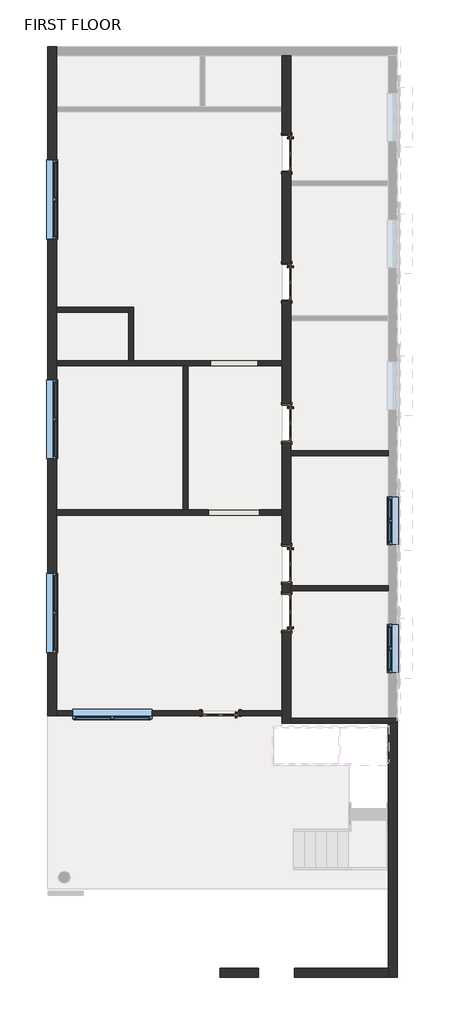
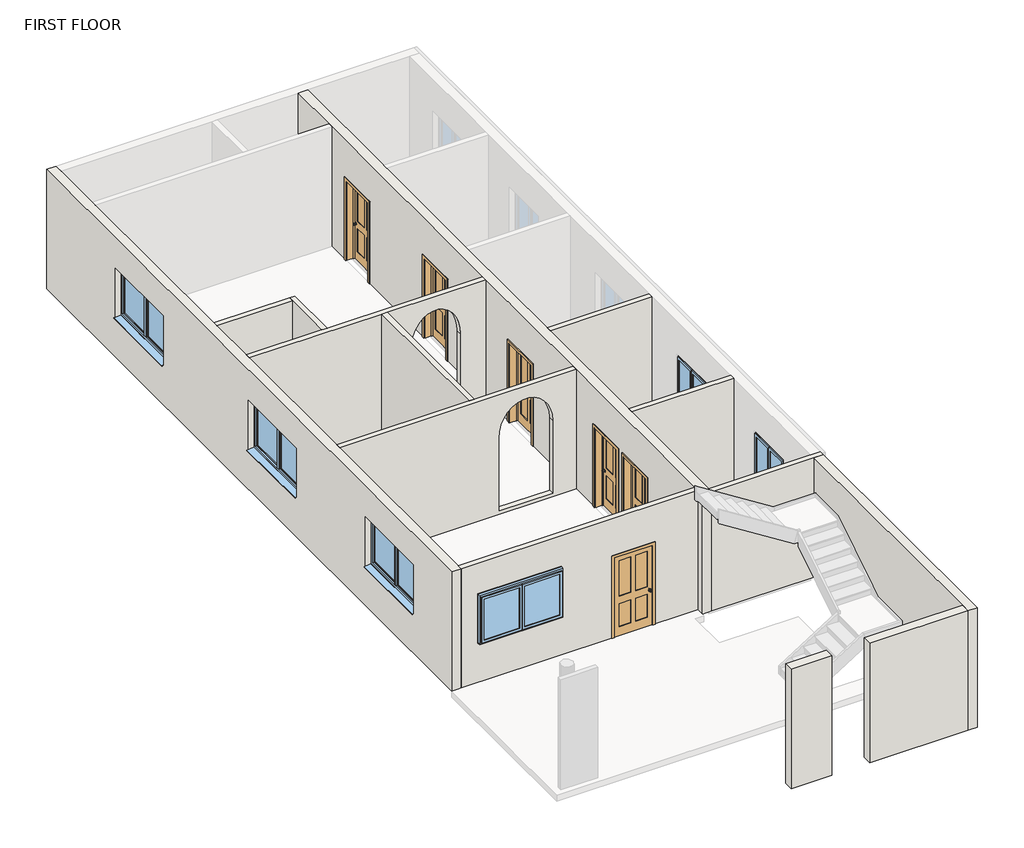
# One storey, part 1 of 2: 13 walls, 6 doors, 6 windows.
"""IFC4 building model written with IfcOpenShell, lengths in millimetres."""

from ifc_helpers import new_model, si_unit, point, frame, origin, place, context, project, spatial, polyline, ellipse_curve, trimmed, outline, extrude, faceted_brep, transform, mapped, element, save
from ifc_brep_helpers import plane_surface, extruded_surface, advanced_brep
from components import door_8a5afc22, door_65ef8926, door_4c85932b, w2_0001_windows_4_x4_9dec5fc7, w2_0001_w2_7b90d420, w2_0001_w2_6e690f8f

model = new_model("IFC4")

# Units and contexts
model_context = context("Model", 3, world=origin())
ifc_project = project(units=[si_unit("LENGTHUNIT", "METRE", prefix="MILLI")], contexts=[model_context])

# Site, building, storey
site = spatial("IfcSite", under=ifc_project)
building = spatial("IfcBuilding", under=site)
storey = spatial("IfcBuildingStorey", under=building, Name="FIRST FLOOR", Elevation=3352.8)

# Doors
placement = place(None, origin())
door_shape = door_8a5afc22(model_context)
element("IfcDoor", 1, ObjectType="Door-Interior-Single-4_Panel-Wood : 36\" x 80\"", at=placement, inside=storey, context=model_context, shape_type="MappedRepresentation", body=[
    mapped(door_shape, transform((7334.4173568, -3037.1073314, 3352.8), x_axis=(0.0, -1.0, 0.0), y_axis=(1.0, 0.0, 0.0), z_axis=(0.0, 0.0, 1.0))),
])
element("IfcDoor", 2, ObjectType="Door-Interior-Single-4_Panel-Wood : 36\" x 80\"", at=placement, inside=storey, context=model_context, shape_type="MappedRepresentation", body=[
    mapped(door_shape, transform((7334.4173568, 531.5926686, 3352.8), x_axis=(0.0, -1.0, 0.0), y_axis=(1.0, 0.0, 0.0), z_axis=(0.0, 0.0, 1.0))),
])
element("IfcDoor", 3, ObjectType="Door-Interior-Single-4_Panel-Wood : 36\" x 80\"", at=placement, inside=storey, context=model_context, shape_type="MappedRepresentation", body=[
    mapped(door_shape, transform((7334.4173568, 4100.2926686, 3352.8), x_axis=(0.0, -1.0, 0.0), y_axis=(1.0, 0.0, 0.0), z_axis=(0.0, 0.0, 1.0))),
])
element("IfcDoor", 4, ObjectType="Door-Interior-Single-4_Panel-Wood : 36\" x 80\"", at=placement, inside=storey, context=model_context, shape_type="MappedRepresentation", body=[
    mapped(door_shape, transform((7334.4173568, 7364.1926686, 3352.8), x_axis=(0.0, -1.0, 0.0), y_axis=(1.0, 0.0, 0.0), z_axis=(0.0, 0.0, 1.0))),
])
door_2_shape = door_65ef8926(model_context)
element("IfcDoor", 5, ObjectType="Door-Interior-Single-4_Panel-Wood : 36\" x 80\"", at=placement, inside=storey, context=model_context, shape_type="MappedRepresentation", body=[
    mapped(door_2_shape, transform((5654.8423568, -6812.1823314, 3352.8), x_axis=(-1.0, 0.0, 0.0), y_axis=(0.0, -1.0, 0.0), z_axis=(0.0, 0.0, 1.0))),
])
door_3_shape = door_4c85932b(model_context)
element("IfcDoor", 6, ObjectType="Door-Interior-Single-4_Panel-Wood : 36\" x 80\"", at=placement, inside=storey, context=model_context, shape_type="MappedRepresentation", body=[
    mapped(door_3_shape, transform((7334.4173568, -4256.3073314, 3352.8), x_axis=(0.0, 1.0, 0.0), y_axis=(-1.0, 0.0, 0.0), z_axis=(0.0, 0.0, 1.0))),
])

# Walls
element("IfcWall", 7, ObjectType="INNER WALL 5\"", at=placement, inside=storey, context=model_context, shape_type="SweptSolid", body=[
    extrude(outline(polyline([(7445.5423568, -166.9073314), (9909.3423568, -166.9073314), (9909.3423568, -293.9073314), (7445.5423568, -293.9073314), (7445.5423568, -166.9073314)])), frame((0.0, 0.0, 3352.8), z_axis=(0.0, 0.0, 1.0), x_axis=(1.0, 0.0, 0.0)), (0.0, 0.0, 1.0), 3048.0),
])
element("IfcWall", 8, ObjectType="INNER WALL 5\"", at=placement, inside=storey, context=model_context, shape_type="SweptSolid", body=[
    extrude(outline(polyline([(7445.5423568, -3583.2073314), (9909.3423568, -3583.2073314), (9909.3423568, -3710.2073314), (7445.5423568, -3710.2073314), (7445.5423568, -3583.2073314)])), frame((0.0, 0.0, 3352.8), z_axis=(0.0, 0.0, 1.0), x_axis=(1.0, 0.0, 0.0)), (0.0, 0.0, 1.0), 3048.0),
])
element("IfcWall", 9, ObjectType="INNER WALL 5\"", at=placement, inside=storey, context=model_context, shape_type="Brep", body=[
    faceted_brep([(7445.5423568, -7063.0073314, 3352.8), (9909.3423568, -7063.0073314, 3352.8), (10137.9423568, -7063.0073314, 3352.8), (10137.9423568, -7063.0073314, 6400.8), (9909.3423568, -7063.0073314, 6400.8), (7445.5423568, -7063.0073314, 6400.8), (7445.5423568, -6936.0073314, 3352.8), (7445.5423568, -6936.0073314, 6400.8), (9909.3423568, -6936.0073314, 6400.8), (10137.9423568, -6936.0073314, 6400.8), (10137.9423568, -6936.0073314, 3352.8), (9909.3423568, -6936.0073314, 3352.8)], [[[0, 1, 2, 3, 4, 5]], [[6, 7, 8, 9, 10, 11]], [[2, 1, 0, 6, 11, 10]], [[5, 4, 3, 9, 8, 7]], [[0, 5, 7, 6]], [[3, 2, 10, 9]]]),
])
element("IfcWall", 10, ObjectType="INNER WALL 5\"", at=placement, inside=storey, context=model_context, shape_type="SweptSolid", body=[
    extrude(outline(polyline([(1501.9423568, 3465.2926686), (3330.7423568, 3465.2926686), (3330.7423568, 3338.2926686), (1501.9423568, 3338.2926686), (1501.9423568, 3465.2926686)])), frame((0.0, 0.0, 3352.8), z_axis=(0.0, 0.0, 1.0), x_axis=(1.0, 0.0, 0.0)), (0.0, 0.0, 1.0), 3048.0),
])
element("IfcWall", 11, ObjectType="INNER WALL 5\"", at=placement, inside=storey, context=model_context, shape_type="AdvancedBrep", body=[
    advanced_brep(
    [(7216.9423568, -1665.5073314, 3352.8), (4829.3423568, -1665.5073314, 3352.8), (4702.3423568, -1665.5073314, 3352.8), (1501.9423568, -1665.5073314, 3352.8), (1501.9423568, -1665.5073314, 6400.8), (4702.3423568, -1665.5073314, 6400.8), (4829.3423568, -1665.5073314, 6400.8), (7216.9423568, -1665.5073314, 6400.8), (5348.459588, -1665.5073314, 3445.3174472), (6643.859588, -1665.5073314, 3445.3174472), (6643.859588, -1665.5073314, 5299.5174472), (5348.459588, -1665.5073314, 5299.5174472), (7216.9423568, -1792.5073314, 3352.8), (7216.9423568, -1792.5073314, 6400.8), (1501.9423568, -1792.5073314, 6400.8), (1501.9423568, -1792.5073314, 3352.8), (5348.459588, -1792.5073314, 3445.3174472), (5348.459588, -1792.5073314, 5299.5174472), (6643.859588, -1792.5073314, 5299.5174472), (6643.859588, -1792.5073314, 3445.3174472)],
    [
        (0, 1),
        (1, 2),
        (2, 3),
        (3, 4),
        (4, 5),
        (5, 6),
        (6, 7),
        (7, 0),
        (8, 9),
        (9, 10),
        (10, 11, ellipse_curve(frame((5996.159588, -1665.5073314, 5299.5174472), z_axis=(0.0, -1.0, 0.0), x_axis=(0.0, 0.0, -1.0)), 787.4, 647.7)),
        (11, 8),
        (12, 13),
        (13, 14),
        (14, 15),
        (15, 12),
        (16, 17),
        (17, 18, ellipse_curve(frame((5996.159588, -1792.5073314, 5299.5174472), z_axis=(0.0, 1.0, 0.0), x_axis=(0.0, 0.0, -1.0)), 787.4, 647.7)),
        (18, 19),
        (19, 16),
        (3, 15),
        (14, 4),
        (7, 13),
        (12, 0),
        (8, 16),
        (19, 9),
        (18, 10),
        (17, 11),
    ],
    [
        plane_surface(frame((7331.2423568, -1665.5073314, 3352.8), z_axis=(0.0, 1.0, 0.0), x_axis=(-1.0, 0.0, 0.0))),
        plane_surface(frame((7331.2423568, -1792.5073314, 3352.8), z_axis=(0.0, -1.0, 0.0), x_axis=(1.0, 0.0, 0.0))),
        plane_surface(frame((1501.9423568, -8333.0073314, 3352.8), z_axis=(-1.0, 0.0, 0.0), x_axis=(0.0, 1.0, 0.0))),
        plane_surface(frame((7216.9423568, 9954.9926686, 3352.8), z_axis=(1.0, 0.0, 0.0), x_axis=(0.0, -1.0, 0.0))),
        plane_surface(frame((7331.2423568, -1665.5073314, 3352.8), z_axis=(0.0, 0.0, -1.0), x_axis=(0.0, -1.0, 0.0))),
        plane_surface(frame((1387.6423568, -1665.5073314, 6400.8), z_axis=(0.0, 0.0, 1.0), x_axis=(0.0, -1.0, 0.0))),
        plane_surface(frame((5348.459588, -1665.5073314, 3445.3174472), z_axis=(0.0, 0.0, 1.0), x_axis=(0.0, -1.0, 0.0))),
        plane_surface(frame((6643.859588, -1665.5073314, 3445.3174472), z_axis=(-1.0, 0.0, 0.0), x_axis=(0.0, -1.0, 0.0))),
        extruded_surface(trimmed(ellipse_curve(frame((5996.159588, -1856.0073314, 5299.5174472), z_axis=(0.0, -1.0, 0.0), x_axis=(-1.0, 0.0, 0.0)), 647.7, 787.4), [point((6643.859588, -1856.0073314, 5299.5174472))], [point((5348.459588, -1856.0073314, 5299.5174472))], True, "CARTESIAN"), (0.0, 127.0, 0.0), 127.0),
        plane_surface(frame((5348.459588, -1665.5073314, 5299.5174472), z_axis=(1.0, 0.0, 0.0), x_axis=(0.0, -1.0, 0.0))),
    ],
    [
        (0, [[1, 2, 3, 4, 5, 6, 7, 8], [9, 10, 11, 12]]),
        (1, [[13, 14, 15, 16], [17, 18, 19, 20]]),
        (2, [[-4, 21, -15, 22]]),
        (3, [[-8, 23, -13, 24]]),
        (4, [[-3, -2, -1, -24, -16, -21]]),
        (5, [[-7, -6, -5, -22, -14, -23]]),
        (6, [[-9, 25, -20, 26]]),
        (7, [[-10, -26, -19, 27]]),
        (8, [[-11, -27, -18, 28]]),
        (9, [[-12, -28, -17, -25]]),
    ],
),
])
element("IfcWall", 12, ObjectType="INNER WALL 5\"", at=placement, inside=storey, context=model_context, shape_type="SweptSolid", body=[
    extrude(outline(polyline([(6400.8, 7216.9423568), (6400.8, 1501.9423568), (3352.8, 1501.9423568), (3352.8, 5172.2423568), (5410.2, 5172.2423568), (5410.2, 6137.4423568), (3352.8, 6137.4423568), (3352.8, 7216.9423568), (6400.8, 7216.9423568)]), holes=[polyline([(5612.8, 3916.6423568), (4352.8, 3916.6423568), (4352.8, 1906.6423568), (5612.8, 1906.6423568), (5612.8, 3916.6423568)])]), frame((0.0, -6872.5073314, 0.0), z_axis=(0.0, 1.0, 0.0), x_axis=(0.0, 0.0, 1.0)), (0.0, 0.0, 1.0), 127.0),
])
element("IfcWall", 13, ObjectType="INNER WALL 5\"", at=placement, inside=storey, context=model_context, shape_type="AdvancedBrep", body=[
    advanced_brep(
    [(1501.9423568, 1992.0926686, 3352.8), (4702.3423568, 1992.0926686, 3352.8), (4829.3423568, 1992.0926686, 3352.8), (7216.9423568, 1992.0926686, 3352.8), (7216.9423568, 1992.0926686, 6400.8), (4829.3423568, 1992.0926686, 6400.8), (4702.3423568, 1992.0926686, 6400.8), (1501.9423568, 1992.0926686, 6400.8), (6599.4941617, 1992.0926686, 3373.8987533), (5405.6941617, 1992.0926686, 3373.8987533), (5405.6941617, 1992.0926686, 5234.4487533), (6599.4941617, 1992.0926686, 5234.4487533), (1501.9423568, 2119.0926686, 3352.8), (1501.9423568, 2119.0926686, 6400.8), (3330.7423568, 2119.0926686, 6400.8), (3457.7423568, 2119.0926686, 6400.8), (7216.9423568, 2119.0926686, 6400.8), (7216.9423568, 2119.0926686, 3352.8), (3457.7423568, 2119.0926686, 3352.8), (3330.7423568, 2119.0926686, 3352.8), (6599.4941617, 2119.0926686, 3373.8987533), (6599.4941617, 2119.0926686, 5234.4487533), (5405.6941617, 2119.0926686, 5234.4487533), (5405.6941617, 2119.0926686, 3373.8987533)],
    [
        (0, 1),
        (1, 2),
        (2, 3),
        (3, 4),
        (4, 5),
        (5, 6),
        (6, 7),
        (7, 0),
        (8, 9),
        (9, 10),
        (10, 11, ellipse_curve(frame((6002.5941617, 1992.0926686, 5234.4487533), z_axis=(0.0, 1.0, 0.0), x_axis=(0.0, 0.0, -1.0)), 812.8, 596.9)),
        (11, 8),
        (12, 13),
        (13, 14),
        (14, 15),
        (15, 16),
        (16, 17),
        (17, 18),
        (18, 19),
        (19, 12),
        (20, 21),
        (21, 22, ellipse_curve(frame((6002.5941617, 2119.0926686, 5234.4487533), z_axis=(0.0, -1.0, 0.0), x_axis=(0.0, 0.0, -1.0)), 812.8, 596.9)),
        (22, 23),
        (23, 20),
        (7, 13),
        (12, 0),
        (3, 17),
        (16, 4),
        (8, 20),
        (23, 9),
        (22, 10),
        (21, 11),
    ],
    [
        plane_surface(frame((1387.6423568, 1992.0926686, 3352.8), z_axis=(0.0, -1.0, 0.0), x_axis=(1.0, 0.0, 0.0))),
        plane_surface(frame((1387.6423568, 2119.0926686, 3352.8), z_axis=(0.0, 1.0, 0.0), x_axis=(-1.0, 0.0, 0.0))),
        plane_surface(frame((1501.9423568, -8333.0073314, 3352.8), z_axis=(-1.0, 0.0, 0.0), x_axis=(0.0, 1.0, 0.0))),
        plane_surface(frame((7216.9423568, 9954.9926686, 3352.8), z_axis=(1.0, 0.0, 0.0), x_axis=(0.0, -1.0, 0.0))),
        plane_surface(frame((1387.6423568, 1992.0926686, 3352.8), z_axis=(0.0, 0.0, -1.0), x_axis=(0.0, 1.0, 0.0))),
        plane_surface(frame((7331.2423568, 1992.0926686, 6400.8), z_axis=(0.0, 0.0, 1.0), x_axis=(0.0, 1.0, 0.0))),
        plane_surface(frame((6599.4941617, 1992.0926686, 3373.8987533), z_axis=(0.0, 0.0, 1.0), x_axis=(0.0, 1.0, 0.0))),
        plane_surface(frame((5405.6941617, 1992.0926686, 3373.8987533), z_axis=(1.0, 0.0, 0.0), x_axis=(0.0, 1.0, 0.0))),
        extruded_surface(trimmed(ellipse_curve(frame((6002.5941617, 2182.5926686, 5234.4487533), z_axis=(0.0, 1.0, 0.0), x_axis=(1.0, 0.0, 0.0)), 596.9, 812.8), [point((5405.6941617, 2182.5926686, 5234.4487533))], [point((6599.4941617, 2182.5926686, 5234.4487533))], True, "CARTESIAN"), (0.0, -127.0, 0.0), 127.0),
        plane_surface(frame((6599.4941617, 1992.0926686, 5234.4487533), z_axis=(-1.0, 0.0, 0.0), x_axis=(0.0, 1.0, 0.0))),
    ],
    [
        (0, [[1, 2, 3, 4, 5, 6, 7, 8], [9, 10, 11, 12]]),
        (1, [[13, 14, 15, 16, 17, 18, 19, 20], [21, 22, 23, 24]]),
        (2, [[-8, 25, -13, 26]]),
        (3, [[-4, 27, -17, 28]]),
        (4, [[-3, -2, -1, -26, -20, -19, -18, -27]]),
        (5, [[-7, -6, -5, -28, -16, -15, -14, -25]]),
        (6, [[-9, 29, -24, 30]]),
        (7, [[-10, -30, -23, 31]]),
        (8, [[-11, -31, -22, 32]]),
        (9, [[-12, -32, -21, -29]]),
    ],
),
])
element("IfcWall", 14, ObjectType="INNER WALL 5\"", at=placement, inside=storey, context=model_context, shape_type="SweptSolid", body=[
    extrude(outline(polyline([(4702.3423568, -1665.5073314), (4702.3423568, 1992.0926686), (4829.3423568, 1992.0926686), (4829.3423568, -1665.5073314), (4702.3423568, -1665.5073314)])), frame((0.0, 0.0, 3352.8), z_axis=(0.0, 0.0, 1.0), x_axis=(1.0, 0.0, 0.0)), (0.0, 0.0, 1.0), 3048.0),
])
element("IfcWall", 15, ObjectType="INNER WALL 5\"", at=placement, inside=storey, context=model_context, shape_type="Brep", body=[
    faceted_brep([(3330.7423568, 3465.2926686, 3352.8), (3330.7423568, 3338.2926686, 3352.8), (3330.7423568, 2119.0926686, 3352.8), (3330.7423568, 2119.0926686, 6400.8), (3330.7423568, 3338.2926686, 6400.8), (3330.7423568, 3465.2926686, 6400.8), (3457.7423568, 3465.2926686, 3352.8), (3457.7423568, 3465.2926686, 6400.8), (3457.7423568, 2119.0926686, 6400.8), (3457.7423568, 2119.0926686, 3352.8)], [[[0, 1, 2, 3, 4, 5]], [[6, 7, 8, 9]], [[2, 1, 0, 6, 9]], [[5, 4, 3, 8, 7]], [[3, 2, 9, 8]], [[0, 5, 7, 6]]]),
])
element("IfcWall", 16, ObjectType="OUTER WALL 9\"", at=placement, inside=storey, context=model_context, shape_type="Brep", body=[
    faceted_brep([(1501.9423568, -6872.5073314, 3352.8), (1501.9423568, -6745.5073314, 3352.8), (1501.9423568, -1792.5073314, 3352.8), (1501.9423568, -1665.5073314, 3352.8), (1501.9423568, 1992.0926686, 3352.8), (1501.9423568, 2119.0926686, 3352.8), (1501.9423568, 3338.2926686, 3352.8), (1501.9423568, 3465.2926686, 3352.8), (1501.9423568, 8418.2926686, 3352.8), (1501.9423568, 8545.2926686, 3352.8), (1501.9423568, 9840.6926686, 3352.8), (1501.9423568, 10069.2926686, 3352.8), (1501.9423568, 10069.2926686, 6400.8), (1501.9423568, 9840.6926686, 6400.8), (1501.9423568, 8545.2926686, 6400.8), (1501.9423568, 8418.2926686, 6400.8), (1501.9423568, 3465.2926686, 6400.8), (1501.9423568, 3338.2926686, 6400.8), (1501.9423568, 2119.0926686, 6400.8), (1501.9423568, 1992.0926686, 6400.8), (1501.9423568, -1665.5073314, 6400.8), (1501.9423568, -1792.5073314, 6400.8), (1501.9423568, -6745.5073314, 6400.8), (1501.9423568, -6872.5073314, 6400.8), (1501.9423568, 5190.7926686, 4352.8), (1501.9423568, 5190.7926686, 5612.8), (1501.9423568, 7200.7926686, 5612.8), (1501.9423568, 7200.7926686, 4352.8), (1501.9423568, -371.8073314, 4352.8), (1501.9423568, -371.8073314, 5612.8), (1501.9423568, 1638.1926686, 5612.8), (1501.9423568, 1638.1926686, 4352.8), (1501.9423568, -5274.0073314, 4352.8), (1501.9423568, -5274.0073314, 5612.8), (1501.9423568, -3264.0073314, 5612.8), (1501.9423568, -3264.0073314, 4352.8), (1273.3423568, -6872.5073314, 3352.8), (1273.3423568, -6872.5073314, 6400.8), (1273.3423568, 10069.2926686, 6400.8), (1273.3423568, 10069.2926686, 3352.8), (1273.3423568, 5190.7926686, 4352.8), (1273.3423568, 7200.7926686, 4352.8), (1273.3423568, 7200.7926686, 5612.8), (1273.3423568, 5190.7926686, 5612.8), (1273.3423568, -371.8073314, 4352.8), (1273.3423568, 1638.1926686, 4352.8), (1273.3423568, 1638.1926686, 5612.8), (1273.3423568, -371.8073314, 5612.8), (1273.3423568, -5274.0073314, 4352.8), (1273.3423568, -3264.0073314, 4352.8), (1273.3423568, -3264.0073314, 5612.8), (1273.3423568, -5274.0073314, 5612.8)], [[[0, 1, 2, 3, 4, 5, 6, 7, 8, 9, 10, 11, 12, 13, 14, 15, 16, 17, 18, 19, 20, 21, 22, 23], [24, 25, 26, 27], [28, 29, 30, 31], [32, 33, 34, 35]], [[36, 37, 38, 39], [40, 41, 42, 43], [44, 45, 46, 47], [48, 49, 50, 51]], [[11, 10, 9, 8, 7, 6, 5, 4, 3, 2, 1, 0, 36, 39]], [[23, 22, 21, 20, 19, 18, 17, 16, 15, 14, 13, 12, 38, 37]], [[12, 11, 39, 38]], [[0, 23, 37, 36]], [[25, 24, 40, 43]], [[26, 25, 43, 42]], [[27, 26, 42, 41]], [[24, 27, 41, 40]], [[29, 28, 44, 47]], [[30, 29, 47, 46]], [[31, 30, 46, 45]], [[28, 31, 45, 44]], [[33, 32, 48, 51]], [[34, 33, 51, 50]], [[35, 34, 50, 49]], [[32, 35, 49, 48]]]),
])
element("IfcWall", 17, ObjectType="OUTER WALL 9\"", at=placement, inside=storey, context=model_context, shape_type="Brep", body=[
    faceted_brep([(7216.9423568, -7063.0073314, 6400.8), (7216.9423568, -6872.5073314, 6400.8), (7216.9423568, -6745.5073314, 6400.8), (7216.9423568, -1792.5073314, 6400.8), (7216.9423568, -1665.5073314, 6400.8), (7216.9423568, 1992.0926686, 6400.8), (7216.9423568, 2119.0926686, 6400.8), (7216.9423568, 8418.2926686, 6400.8), (7216.9423568, 8545.2926686, 6400.8), (7216.9423568, 9840.6926686, 6400.8), (7216.9423568, 9840.6926686, 3352.8), (7216.9423568, 8545.2926686, 3352.8), (7216.9423568, 8418.2926686, 3352.8), (7216.9423568, 7846.7926686, 3352.8), (7216.9423568, 7846.7926686, 5410.2), (7216.9423568, 6881.5926686, 5410.2), (7216.9423568, 6881.5926686, 3352.8), (7216.9423568, 4582.8926686, 3352.8), (7216.9423568, 4582.8926686, 5410.2), (7216.9423568, 3617.6926686, 5410.2), (7216.9423568, 3617.6926686, 3352.8), (7216.9423568, 2119.0926686, 3352.8), (7216.9423568, 1992.0926686, 3352.8), (7216.9423568, 1014.1926686, 3352.8), (7216.9423568, 1014.1926686, 5410.2), (7216.9423568, 48.9926686, 5410.2), (7216.9423568, 48.9926686, 3352.8), (7216.9423568, -1665.5073314, 3352.8), (7216.9423568, -1792.5073314, 3352.8), (7216.9423568, -2554.5073314, 3352.8), (7216.9423568, -2554.5073314, 5410.2), (7216.9423568, -3519.7073314, 5410.2), (7216.9423568, -3519.7073314, 3352.8), (7216.9423568, -3773.7073314, 3352.8), (7216.9423568, -3773.7073314, 5410.2), (7216.9423568, -4738.9073314, 5410.2), (7216.9423568, -4738.9073314, 3352.8), (7216.9423568, -6745.5073314, 3352.8), (7216.9423568, -6872.5073314, 3352.8), (7216.9423568, -7063.0073314, 3352.8), (7445.5423568, 9840.6926686, 6400.8), (7445.5423568, 6665.6926686, 6400.8), (7445.5423568, 6538.6926686, 6400.8), (7445.5423568, 3249.3926686, 6400.8), (7445.5423568, 3122.3926686, 6400.8), (7445.5423568, -166.9073314, 6400.8), (7445.5423568, -293.9073314, 6400.8), (7445.5423568, -3583.2073314, 6400.8), (7445.5423568, -3710.2073314, 6400.8), (7445.5423568, -6936.0073314, 6400.8), (7445.5423568, -7063.0073314, 6400.8), (7445.5423568, -7063.0073314, 3352.8), (7445.5423568, -6936.0073314, 3352.8), (7445.5423568, -4738.9073314, 3352.8), (7445.5423568, -4738.9073314, 5410.2), (7445.5423568, -3773.7073314, 5410.2), (7445.5423568, -3773.7073314, 3352.8), (7445.5423568, -3710.2073314, 3352.8), (7445.5423568, -3583.2073314, 3352.8), (7445.5423568, -3519.7073314, 3352.8), (7445.5423568, -3519.7073314, 5410.2), (7445.5423568, -2554.5073314, 5410.2), (7445.5423568, -2554.5073314, 3352.8), (7445.5423568, -293.9073314, 3352.8), (7445.5423568, -166.9073314, 3352.8), (7445.5423568, 48.9926686, 3352.8), (7445.5423568, 48.9926686, 5410.2), (7445.5423568, 1014.1926686, 5410.2), (7445.5423568, 1014.1926686, 3352.8), (7445.5423568, 3122.3926686, 3352.8), (7445.5423568, 3249.3926686, 3352.8), (7445.5423568, 3617.6926686, 3352.8), (7445.5423568, 3617.6926686, 5410.2), (7445.5423568, 4582.8926686, 5410.2), (7445.5423568, 4582.8926686, 3352.8), (7445.5423568, 6538.6926686, 3352.8), (7445.5423568, 6665.6926686, 3352.8), (7445.5423568, 6881.5926686, 3352.8), (7445.5423568, 6881.5926686, 5410.2), (7445.5423568, 7846.7926686, 5410.2), (7445.5423568, 7846.7926686, 3352.8), (7445.5423568, 9840.6926686, 3352.8)], [[[0, 1, 2, 3, 4, 5, 6, 7, 8, 9, 10, 11, 12, 13, 14, 15, 16, 17, 18, 19, 20, 21, 22, 23, 24, 25, 26, 27, 28, 29, 30, 31, 32, 33, 34, 35, 36, 37, 38, 39]], [[40, 41, 42, 43, 44, 45, 46, 47, 48, 49, 50, 51, 52, 53, 54, 55, 56, 57, 58, 59, 60, 61, 62, 63, 64, 65, 66, 67, 68, 69, 70, 71, 72, 73, 74, 75, 76, 77, 78, 79, 80, 81]], [[10, 81, 80, 13, 12, 11]], [[51, 39, 38, 37, 36, 53, 52]], [[16, 77, 76, 75, 74, 17]], [[20, 71, 70, 69, 68, 23, 22, 21]], [[26, 65, 64, 63, 62, 29, 28, 27]], [[32, 59, 58, 57, 56, 33]], [[9, 8, 7, 6, 5, 4, 3, 2, 1, 0, 50, 49, 48, 47, 46, 45, 44, 43, 42, 41, 40]], [[10, 9, 40, 81]], [[0, 39, 51, 50]], [[15, 78, 77, 16]], [[78, 15, 14, 79]], [[79, 14, 13, 80]], [[19, 72, 71, 20]], [[72, 19, 18, 73]], [[73, 18, 17, 74]], [[25, 66, 65, 26]], [[66, 25, 24, 67]], [[67, 24, 23, 68]], [[31, 60, 59, 32]], [[60, 31, 30, 61]], [[61, 30, 29, 62]], [[55, 34, 33, 56]], [[34, 55, 54, 35]], [[35, 54, 53, 36]]]),
])
element("IfcWall", 18, ObjectType="OUTER WALL 9\"", at=placement, inside=storey, context=model_context, shape_type="Brep", body=[
    faceted_brep([(9909.3423568, -7063.0073314, 3352.8), (9909.3423568, -13273.3073314, 3352.8), (9909.3423568, -13501.9073314, 3352.8), (9909.3423568, -13501.9073314, 6400.8), (9909.3423568, -13273.3073314, 6400.8), (9909.3423568, -7063.0073314, 6400.8), (10137.9423568, -7063.0073314, 3352.8), (10137.9423568, -7063.0073314, 6400.8), (10137.9423568, -13501.9073314, 6400.8), (10137.9423568, -13501.9073314, 3352.8)], [[[0, 1, 2, 3, 4, 5]], [[6, 7, 8, 9]], [[2, 1, 0, 6, 9]], [[5, 4, 3, 8, 7]], [[0, 5, 7, 6]], [[3, 2, 9, 8]]]),
])
element("IfcWall", 19, ObjectType="OUTER WALL 9\"", at=placement, inside=storey, context=model_context, shape_type="SweptSolid", body=[
    extrude(outline(polyline([(5642.1423568, -13501.9073314), (5642.1423568, -13273.3073314), (6619.47371, -13273.3073314), (6619.47371, -13501.9073314), (5642.1423568, -13501.9073314)])), frame((0.0, 0.0, 3352.8), z_axis=(0.0, 0.0, 1.0), x_axis=(1.0, 0.0, 0.0)), (0.0, 0.0, 1.0), 3048.0),
    extrude(outline(polyline([(9909.3423568, -13273.3073314), (9909.3423568, -13501.9073314), (7533.87371, -13501.9073314), (7533.87371, -13273.3073314), (9909.3423568, -13273.3073314)])), frame((0.0, 0.0, 3352.8), z_axis=(0.0, 0.0, 1.0), x_axis=(1.0, 0.0, 0.0)), (0.0, 0.0, 1.0), 3048.0),
])

# Windows
w2_0001_windows_4_x4_shape = w2_0001_windows_4_x4_9dec5fc7(model_context)
element("IfcWindow", 20, ObjectType="w2.0001 : WINDOWS 4' X4'", at=placement, inside=storey, context=model_context, shape_type="MappedRepresentation", body=[
    mapped(w2_0001_windows_4_x4_shape, transform((10023.6423568, -1938.5573314, 3352.8), x_axis=(0.0, -1.0, 0.0), y_axis=(1.0, 0.0, 0.0), z_axis=(0.0, 0.0, 1.0))),
])
element("IfcWindow", 21, ObjectType="w2.0001 : WINDOWS 4' X4'", at=placement, inside=storey, context=model_context, shape_type="MappedRepresentation", body=[
    mapped(w2_0001_windows_4_x4_shape, transform((10023.6423568, -5170.7073314, 3352.8), x_axis=(0.0, -1.0, 0.0), y_axis=(1.0, 0.0, 0.0), z_axis=(0.0, 0.0, 1.0))),
])
w2_0001_w2_shape = w2_0001_w2_7b90d420(model_context)
element("IfcWindow", 22, ObjectType="w2.0001 : w2", at=placement, inside=storey, context=model_context, shape_type="MappedRepresentation", body=[
    mapped(w2_0001_w2_shape, transform((1387.6423568, -4269.0073314, 3352.8), x_axis=(0.0, 1.0, 0.0), y_axis=(-1.0, 0.0, 0.0), z_axis=(0.0, 0.0, 1.0))),
])
element("IfcWindow", 23, ObjectType="w2.0001 : w2", at=placement, inside=storey, context=model_context, shape_type="MappedRepresentation", body=[
    mapped(w2_0001_w2_shape, transform((1387.6423568, 633.1926686, 3352.8), x_axis=(0.0, 1.0, 0.0), y_axis=(-1.0, 0.0, 0.0), z_axis=(0.0, 0.0, 1.0))),
])
element("IfcWindow", 24, ObjectType="w2.0001 : w2", at=placement, inside=storey, context=model_context, shape_type="MappedRepresentation", body=[
    mapped(w2_0001_w2_shape, transform((1387.6423568, 6195.7926686, 3352.8), x_axis=(0.0, 1.0, 0.0), y_axis=(-1.0, 0.0, 0.0), z_axis=(0.0, 0.0, 1.0))),
])
w2_0001_w2_2_shape = w2_0001_w2_6e690f8f(model_context)
element("IfcWindow", 25, ObjectType="w2.0001 : w2", at=placement, inside=storey, context=model_context, shape_type="MappedRepresentation", body=[
    mapped(w2_0001_w2_2_shape, transform((2911.6423568, -6809.0073314, 3352.8), x_axis=(-1.0, 0.0, 0.0), y_axis=(0.0, -1.0, 0.0), z_axis=(0.0, 0.0, 1.0))),
])

save(model, "model.ifc")

# Revit data of these elements
# Type "Door-Interior-Single-4_Panel-Wood : 36\" x 80\""
#   Type Mark = "9"
#   Assembly Code = "C1020300"
#   Analytic Construction = "Wooden"
#   Top Rail = 0' - 4 11/16"
#   Thickness = 0' - 1 3/8"
#   Thermal Resistance (R) = 2.5876 (h·ft²·°F)/BTU
#   Swing Angle [instance default] = 90.00°
#   Stiles = 0' - 4 3/4"
#   Rough Width = 3' - 2"
#   Rough Height = 6' - 9"
#   Mullion = 0' - 4 1/2"
#   Lock Rail = 0' - 7 1/2"
#   Height = 6' - 8"
#   Width = 3' - 0"
#   Heat Transfer Coefficient (U) = 0.3865 BTU/(h·ft²·°F)
#   Bottom Rail = 0' - 9 1/8"
#   Trim Material = Cherry
#   Panel Material = Cherry
#   Frame Material = Cherry
#   Door Handle Material = Aluminum
#   Visual Light Transmittance = 0
#   Solar Heat Gain Coefficient = 0
#   Wall Closure = (empty or 0)
#   Function = (empty or 0)
# Type "INNER WALL 5\""
#   Assembly Code = "B2010"
#   Layers, outside or top first: 0' - 5" "CREAM BEIGE COLOUR" (function 1)
# Type "OUTER WALL 9\""
#   Assembly Code = "B2010"
#   Layers, outside or top first: 0' - 9" "CREAM BEIGE COLOUR" (function 1)
# Type "w2.0001 : WINDOWS 4' X4'"
#   Type Mark = "22"
#   Operation = "DoublePanelVertical"
#   Keynote = "16.05.01"
#   Analytic Construction = "<None>"
#   Rough Width = 4' - 0"
#   Rough Height = 4' - 0"
#   Rahmentiefe = 0' - 2.3622"
#   Rahmenhöhe unten = 0' - 3.14961"
#   Rahmehöhe oben = 0' - 3.14961"
#   Rahmenbreite = 0' - 2.3622"
#   Height = 4' - 0"
#   Flügeltiefe = 0' - 2.3622"
#   Flügelbreite = 0' - 2.3622"
#   Einbautiefe (von außen) [instance default] = 0' - 5.51181"
#   Width = 4' - 0"
#   Kippflügel [instance default] = yes
#   Drehflügel im Grundriß darstellen [instance default] = no
#   Drehflügel [instance default] = yes
#   Define Thermal Properties by = 1
#   Rahmen [instance default] = none
#   Glas [instance default] = none
#   Flügel [instance default] = none
#   Fensterbank aussen [instance default] = none
#   Fensterbank innen [instance default] = none
#   Wall Closure = (empty or 0)
# Type "w2.0001 : w2"
#   Type Mark = "19"
#   Operation = "DoublePanelVertical"
#   Keynote = "16.05.01"
#   Analytic Construction = "<None>"
#   Rough Width = 6' - 7.13386"
#   Rough Height = 4' - 1.6063"
#   Rahmentiefe = 0' - 2.3622"
#   Rahmenhöhe unten = 0' - 3.14961"
#   Rahmehöhe oben = 0' - 3.14961"
#   Rahmenbreite = 0' - 2.3622"
#   Height = 4' - 1.6063"
#   Flügeltiefe = 0' - 2.3622"
#   Flügelbreite = 0' - 2.3622"
#   Einbautiefe (von außen) [instance default] = 0' - 5.51181"
#   Width = 6' - 7.13386"
#   Kippflügel [instance default] = yes
#   Drehflügel im Grundriß darstellen [instance default] = no
#   Drehflügel [instance default] = yes
#   Define Thermal Properties by = 1
#   Rahmen [instance default] = none
#   Glas [instance default] = none
#   Flügel [instance default] = none
#   Fensterbank aussen [instance default] = none
#   Fensterbank innen [instance default] = none
#   Wall Closure = (empty or 0)
# Elements 1, 2, 3, 4, 5, 6 (IfcDoor, "Door-Interior-Single-4_Panel-Wood : 36\" x 80\"")
#   Swing Angle = 90.00°
#   Phase Created = New Construction
#   Materials on its faces: "Cherry", "Aluminum"
# Elements 7, 8, 9, 10, 11, 12, 13, 14, 15 (IfcWall, "INNER WALL 5\"")
#   Top Offset = 0' - 0"
#   Base Offset = 0' - 0"
#   wall height = 10' - 0"
#   Phase Created = New Construction
#   Base Constraint = FIRST FLOOR
#   Top Constraint = Level 4
#   Materials on its faces: "CREAM BEIGE COLOUR"
# Elements 16, 17 (IfcWall, "OUTER WALL 9\"")
#   Top Offset = 0' - 0"
#   Base Offset = 0' - 0"
#   Unconnected Height = 10' - 0"
#   wall height = 10' - 0"
#   Phase Created = New Construction
#   Base Constraint = FIRST FLOOR
#   Materials on its faces: "CREAM BEIGE COLOUR"
# Elements 18, 19 (IfcWall, "OUTER WALL 9\"")
#   Top Offset = 0' - 0"
#   Base Offset = 0' - 0"
#   wall height = 10' - 0"
#   Phase Created = New Construction
#   Base Constraint = FIRST FLOOR
#   Top Constraint = Level 4
#   Materials on its faces: "CREAM BEIGE COLOUR"
# Element 20 (IfcWindow, "w2.0001 : WINDOWS 4' X4'")
#   Mark = "9"
#   Einbautiefe (von außen) = 0' - 5.51181"
#   Kippflügel = yes
#   Drehflügel im Grundriß darstellen = no
#   Drehflügel = yes
#   Rahmen = none
#   Glas = none
#   Flügel = none
#   Fensterbank innen = none
#   Fensterbank aussen = none
#   Phase Created = New Construction
#   Materials on its faces: "Fenster - Kunststoff", "Fenster - Kunststoff weiss", "Glass", "Fenster - Holz"
# Element 21 (IfcWindow, "w2.0001 : WINDOWS 4' X4'")
#   Mark = "13"
#   Einbautiefe (von außen) = 0' - 5.51181"
#   Kippflügel = yes
#   Drehflügel im Grundriß darstellen = no
#   Drehflügel = yes
#   Rahmen = none
#   Glas = none
#   Flügel = none
#   Fensterbank innen = none
#   Fensterbank aussen = none
#   Phase Created = New Construction
#   Materials on its faces: "Fenster - Kunststoff", "Fenster - Kunststoff weiss", "Glass", "Fenster - Holz"
# Element 22 (IfcWindow, "w2.0001 : w2")
#   Mark = "6"
#   Einbautiefe (von außen) = 0' - 5.51181"
#   Kippflügel = yes
#   Drehflügel im Grundriß darstellen = no
#   Drehflügel = yes
#   Rahmen = none
#   Glas = none
#   Flügel = none
#   Fensterbank innen = none
#   Fensterbank aussen = none
#   Phase Created = New Construction
#   Materials on its faces: "Fenster - Kunststoff", "Fenster - Kunststoff weiss", "Glass", "Fenster - Holz"
# Element 23 (IfcWindow, "w2.0001 : w2")
#   Mark = "7"
#   Einbautiefe (von außen) = 0' - 5.51181"
#   Kippflügel = yes
#   Drehflügel im Grundriß darstellen = no
#   Drehflügel = yes
#   Rahmen = none
#   Glas = none
#   Flügel = none
#   Fensterbank innen = none
#   Fensterbank aussen = none
#   Phase Created = New Construction
#   Materials on its faces: "Fenster - Kunststoff", "Fenster - Kunststoff weiss", "Glass", "Fenster - Holz"
# Element 24 (IfcWindow, "w2.0001 : w2")
#   Mark = "8"
#   Einbautiefe (von außen) = 0' - 5.51181"
#   Kippflügel = yes
#   Drehflügel im Grundriß darstellen = no
#   Drehflügel = yes
#   Rahmen = none
#   Glas = none
#   Flügel = none
#   Fensterbank innen = none
#   Fensterbank aussen = none
#   Phase Created = New Construction
#   Materials on its faces: "Fenster - Kunststoff", "Fenster - Kunststoff weiss", "Glass", "Fenster - Holz"
# Element 25 (IfcWindow, "w2.0001 : w2")
#   Mark = "5"
#   Einbautiefe (von außen) = 0' - 5.51181"
#   Kippflügel = yes
#   Drehflügel im Grundriß darstellen = no
#   Drehflügel = yes
#   Rahmen = none
#   Glas = none
#   Flügel = none
#   Fensterbank innen = none
#   Fensterbank aussen = none
#   Phase Created = New Construction
#   Materials on its faces: "Fenster - Kunststoff", "Fenster - Kunststoff weiss", "Glass", "Fenster - Holz"
# Materials
#   "Cherry": class "Wood", colour RGB 226 177 128, transparency 0, Description = "Prunus Serotina", Cost = 0
#   "Aluminum": class "Metal", colour RGB 247 247 247, transparency 0, Description = "Aluminum 6061", Cost = 0
#   "CREAM BEIGE COLOUR": class "Generic", colour RGB 120 120 120, transparency 0, Cost = 0
#   "Fenster - Kunststoff": colour RGB 249 249 249, transparency 0
#   "Fenster - Kunststoff weiss": colour RGB 249 249 249, transparency 0
#   "Glass": class "Glass", colour RGB 0 128 192, transparency 0.75, Description = "Soda Lime Glass", Cost = 0
#   "Fenster - Holz": colour RGB 216 135 75, transparency 0
